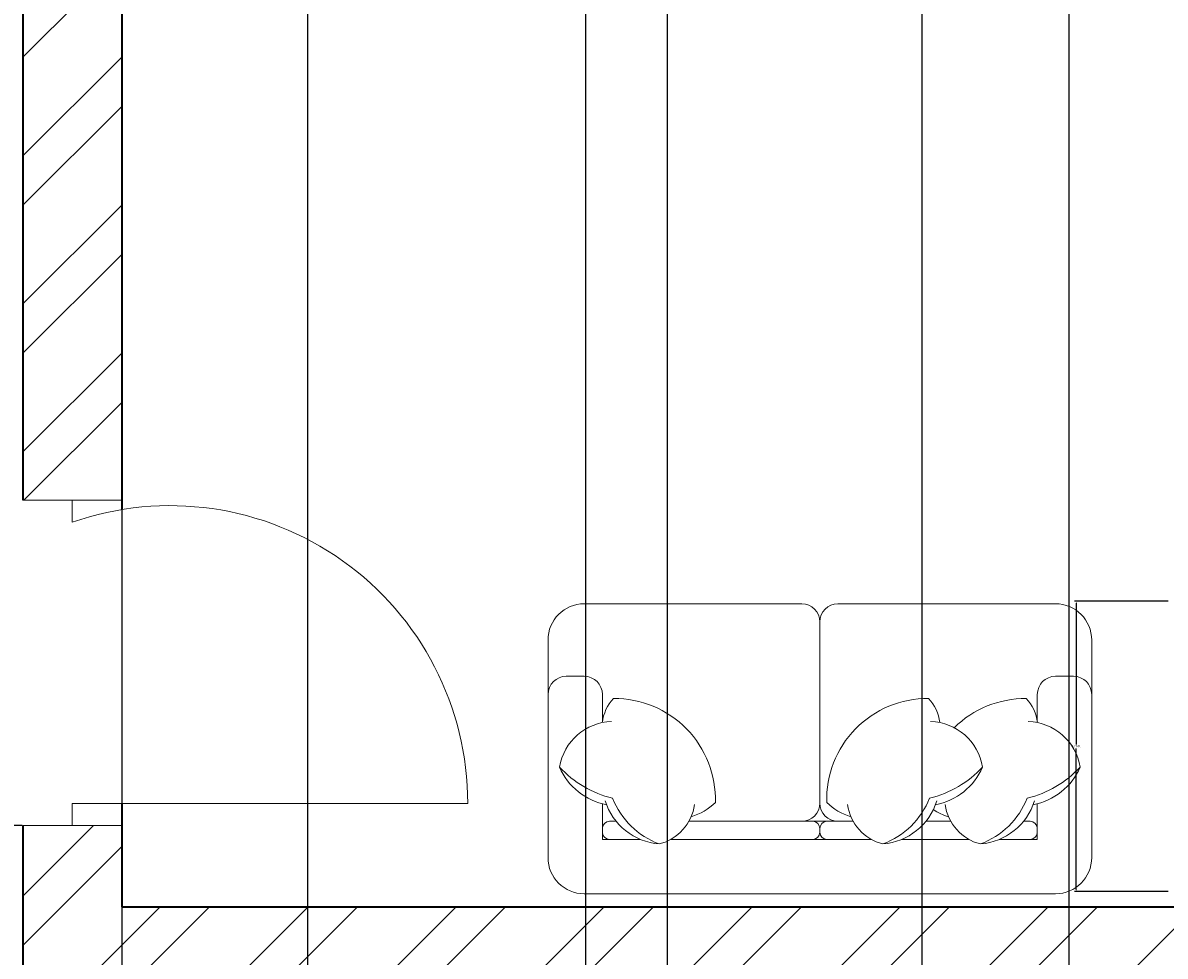
# Model space of a CAD drawing. Units: inches. Extents: x 2552 to 3217, y 1417 to 2737.
# Tile 20 of 25: x 2909 to 3013, y 2392 to 2476. Entities that reach past the tile are written whole.
import ezdxf

# ---------------------------------------------------------------- set-up
doc = ezdxf.new("R2010")
doc.units = ezdxf.units.IN
for name, color, linetype, lineweight in [('A-ANNO-DIMS', 2, 'Continuous', 18), ('A-DOOR', 21, 'Continuous', 18), ('A-FURN', 8, 'Continuous', 13), ('A-WALL', 7, 'Continuous', 35), ('A-WALL-PATT', 217, 'Continuous', 13)]:
    doc.layers.add(name, color=color, linetype=linetype, lineweight=lineweight)
doc.styles.get("Standard").update_dxf_attribs({"font": 'arial.ttf'})
doc.dimstyles.get("Standard").update_dxf_attribs({"dimtxt": 0.18, "dimasz": 0.18, "dimexe": 0.18, "dimexo": 0.0625, "dimgap": 0.09, "dimtad": 0, "dimtih": 1, "dimtoh": 1, "dimdec": 4, "dimzin": 0, "dimdsep": 46, "dimtxsty": 'Standard', "dimcen": 0.09, "dimadec": 0, "dimazin": 0, "dimtfac": 1, "dimtdec": 4, "dimtofl": 0, "dimtmove": 0, "dimatfit": 3, "dimfxl": 1, "dimtolj": 1, "dimtzin": 0, "dimarcsym": 0})

# ---------------------------------------------------------------- blocks, each defined once
blk = doc.blocks.new('*D46')
at = {"layer": 'A-ANNO-DIMS', "color": 0, "lineweight": -2, "transparency": 16777216}
for p, q in [((3013.1, 2423.8), (3004.57, 2423.8)), ((3004.75, 2423.62), (3004.75, 2410.78)), ((3004.75, 2397.59), (3004.75, 2410.42)), ((3013.1, 2397.41), (3004.57, 2397.41))]:
    blk.add_line(p, q, dxfattribs=at)
at = {"layer": 'A-ANNO-DIMS', "color": 0, "transparency": 16777216}
for points in [[(3004.72, 2423.62), (3004.78, 2423.62), (3004.75, 2423.8)], [(3004.72, 2397.59), (3004.78, 2397.59), (3004.75, 2397.41)]]:
    blk.add_solid(points, dxfattribs=at)
at = {"layer": 'Defpoints', "color": 0, "transparency": 16777216}
for p in [(3004.75, 2423.8), (3013.16, 2423.8), (3013.16, 2397.41)]:
    blk.add_point(p, dxfattribs=at)
at = {"layer": 'A-ANNO-DIMS', "color": 0, "transparency": 16777216, "insert": (3004.75, 2410.6), "char_height": 0.18, "attachment_point": 5}
blk.add_mtext('\\A1;26 TYP.', dxfattribs=at)
blk = doc.blocks.new('*D56')
at = {"layer": 'A-ANNO-DIMS', "color": 0, "lineweight": -2, "transparency": 16777216}
for p, q in [((2967.49, 2515.95), (2967.49, 1482.53)), ((2990.69, 2515.95), (2990.69, 1482.53)), ((2967.67, 1482.71), (2978.76, 1482.71)), ((2990.51, 1482.71), (2979.41, 1482.71))]:
    blk.add_line(p, q, dxfattribs=at)
at = {"layer": 'A-ANNO-DIMS', "color": 0, "transparency": 16777216}
for points in [[(2967.67, 1482.74), (2967.67, 1482.68), (2967.49, 1482.71)], [(2990.51, 1482.74), (2990.51, 1482.68), (2990.69, 1482.71)]]:
    blk.add_solid(points, dxfattribs=at)
at = {"layer": 'Defpoints', "color": 0, "transparency": 16777216}
for p in [(2967.49, 2516.01), (2990.69, 2516.01), (2990.69, 1482.71)]:
    blk.add_point(p, dxfattribs=at)
at = {"layer": 'A-ANNO-DIMS', "color": 0, "transparency": 16777216, "insert": (2979.09, 1482.71), "char_height": 0.18, "attachment_point": 5}
blk.add_mtext('\\A1;23.2', dxfattribs=at)
blk = doc.blocks.new('*D57')
at = {"layer": 'A-ANNO-DIMS', "color": 0, "lineweight": -2, "transparency": 16777216}
for p, q in [((3004.08, 2515.95), (3004.08, 1482.53)), ((3036.34, 2515.95), (3036.34, 1482.53)), ((3004.26, 1482.71), (3019.75, 1482.71)), ((3036.16, 1482.71), (3020.68, 1482.71))]:
    blk.add_line(p, q, dxfattribs=at)
at = {"layer": 'A-ANNO-DIMS', "color": 0, "transparency": 16777216}
for points in [[(3004.26, 1482.74), (3004.26, 1482.68), (3004.08, 1482.71)], [(3036.16, 1482.74), (3036.16, 1482.68), (3036.34, 1482.71)]]:
    blk.add_solid(points, dxfattribs=at)
at = {"layer": 'Defpoints', "color": 0, "transparency": 16777216}
for p in [(3004.08, 2516.01), (3036.34, 2516.01), (3036.34, 1482.71)]:
    blk.add_point(p, dxfattribs=at)
at = {"layer": 'A-ANNO-DIMS', "color": 0, "transparency": 16777216, "insert": (3020.21, 1482.71), "char_height": 0.18, "attachment_point": 5}
blk.add_mtext('\\A1;32.255', dxfattribs=at)
blk = doc.blocks.new('*D64')
at = {"layer": 'A-ANNO-DIMS', "color": 0, "lineweight": -2, "transparency": 16777216}
for p, q in [((2646.35, 1551.58), (2646.35, 2709.49)), ((2646.53, 2709.31), (2802.77, 2709.31)), ((2959.93, 2709.31), (2803.69, 2709.31)), ((2960.11, 1551.58), (2960.11, 2709.49))]:
    blk.add_line(p, q, dxfattribs=at)
at = {"layer": 'A-ANNO-DIMS', "color": 0, "transparency": 16777216}
for points in [[(2646.53, 2709.34), (2646.53, 2709.28), (2646.35, 2709.31)], [(2959.93, 2709.34), (2959.93, 2709.28), (2960.11, 2709.31)]]:
    blk.add_solid(points, dxfattribs=at)
at = {"layer": 'Defpoints', "color": 0, "transparency": 16777216}
for p in [(2960.11, 2709.31), (2646.35, 1551.51), (2960.11, 1551.51)]:
    blk.add_point(p, dxfattribs=at)
at = {"layer": 'A-ANNO-DIMS', "color": 0, "transparency": 16777216, "insert": (2803.23, 2709.31), "char_height": 0.18, "attachment_point": 5}
blk.add_mtext('\\A1;313.76', dxfattribs=at)
blk = doc.blocks.new('*D67')
at = {"layer": 'A-ANNO-DIMS', "color": 0, "lineweight": -2, "transparency": 16777216}
for p, q in [((2917.85, 2640.45), (2917.85, 1482.53)), ((2934.77, 2624.73), (2934.77, 1482.53)), ((2918.03, 1482.71), (2925.86, 1482.71)), ((2934.59, 1482.71), (2926.76, 1482.71))]:
    blk.add_line(p, q, dxfattribs=at)
at = {"layer": 'A-ANNO-DIMS', "color": 0, "transparency": 16777216}
for points in [[(2918.03, 1482.74), (2918.03, 1482.68), (2917.85, 1482.71)], [(2934.59, 1482.74), (2934.59, 1482.68), (2934.77, 1482.71)]]:
    blk.add_solid(points, dxfattribs=at)
at = {"layer": 'Defpoints', "color": 0, "transparency": 16777216}
for p in [(2917.85, 2640.51), (2934.77, 2624.79), (2934.77, 1482.71)]:
    blk.add_point(p, dxfattribs=at)
at = {"layer": 'A-ANNO-DIMS', "color": 0, "transparency": 16777216, "insert": (2926.31, 1482.71), "char_height": 0.18, "attachment_point": 5}
blk.add_mtext('\\A1;16.912', dxfattribs=at)
blk = doc.blocks.new('*D69')
at = {"layer": 'A-ANNO-DIMS', "color": 0, "lineweight": -2, "transparency": 16777216}
for p, q in [((2908.79, 2403.41), (2577.37, 2403.41)), ((2577.55, 2403.23), (2577.55, 2395.39)), ((2577.55, 2387.19), (2577.55, 2395.03)), ((2917.79, 2387.01), (2577.37, 2387.01))]:
    blk.add_line(p, q, dxfattribs=at)
at = {"layer": 'A-ANNO-DIMS', "color": 0, "transparency": 16777216}
for points in [[(2577.52, 2403.23), (2577.58, 2403.23), (2577.55, 2403.41)], [(2577.52, 2387.19), (2577.58, 2387.19), (2577.55, 2387.01)]]:
    blk.add_solid(points, dxfattribs=at)
at = {"layer": 'Defpoints', "color": 0, "transparency": 16777216}
for p in [(2577.55, 2403.41), (2908.85, 2403.41), (2917.85, 2387.01)]:
    blk.add_point(p, dxfattribs=at)
at = {"layer": 'A-ANNO-DIMS', "color": 0, "transparency": 16777216, "insert": (2577.55, 2395.21), "char_height": 0.18, "attachment_point": 5}
blk.add_mtext('\\A1;16.4', dxfattribs=at)

msp = doc.modelspace()

# ---------------------------------------------------------------- hatches: boundary and pattern name
at = {"layer": 'A-WALL-PATT'}
h = msp.add_hatch(dxfattribs=at)
h.set_pattern_fill('ANSI32', color=256)
h.paths.add_polyline_path([(2756.676, 2649.5125), (2637.3535, 2649.5125), (2637.3535, 2617.9626), (2641.8535, 2617.9626), (2646.3535, 2617.9626), (2646.3535, 2640.5125), (2724.3535, 2640.5125), (2724.3535, 2520.5125), (2720.299, 2520.5125), (2720.299, 2516.0125), (2733.4075, 2516.0125), (2733.4075, 2518.2213), (2733.4075, 2520.5125), (2728.8535, 2520.5125), (2728.8535, 2640.5125), (2756.676, 2640.5125)])
h.paths.add_polyline_path([(2848.8535, 2649.5125), (2804.676, 2649.5125), (2804.676, 2640.5125), (2839.8535, 2640.5125), (2839.8535, 2598.3517), (2848.8535, 2598.3517)])
h.paths.add_polyline_path([(2646.3535, 2516.0125), (2697.9593, 2516.0125), (2697.9593, 2518.2625), (2697.9593, 2520.5125), (2646.3535, 2520.5125), (2646.3535, 2581.9626), (2637.3535, 2581.9626), (2637.3535, 2364.3298), (2646.3535, 2364.3298), (2646.3535, 2387.0125), (2724.3535, 2387.0125), (2724.3535, 2267.0125), (2721.0443, 2267.0125), (2721.0443, 2262.5125), (2733.7854, 2262.5125), (2733.7854, 2264.7625), (2733.7854, 2267.0125), (2728.8535, 2267.0125), (2728.8535, 2387.0125), (2839.8535, 2387.0125), (2839.8535, 2363.8387), (2848.8535, 2363.8387), (2848.8535, 2403.7415), (2844.3535, 2403.7415), (2839.8535, 2403.7415), (2839.8535, 2396.0125), (2646.3535, 2396.0125)])
h.paths.add_polyline_path([(2848.8535, 2550.3517), (2844.3535, 2550.3517), (2839.8535, 2550.3517), (2839.8535, 2520.5125), (2801.9195, 2520.5125), (2801.9195, 2518.2625), (2801.9195, 2516.0125), (2839.8535, 2516.0125), (2839.8535, 2507.5813), (2848.8535, 2507.5813)], flags=17)
h.paths.add_polyline_path([(2848.8535, 2483.5813), (2844.3535, 2483.5813), (2839.8535, 2483.5813), (2839.8535, 2468.0125), (2773.8535, 2468.0125), (2773.8535, 2516.0125), (2778.1336, 2516.0125), (2778.1336, 2520.5125), (2766.696, 2520.5125), (2766.696, 2518.2625), (2766.696, 2516.0125), (2769.3535, 2516.0125), (2769.3535, 2463.5125), (2839.8535, 2463.5125), (2839.8535, 2431.0782), (2848.8535, 2431.0782)], flags=17)
h.paths.add_polyline_path([(2917.8535, 2569.2764), (2913.3535, 2569.2764), (2908.8535, 2569.2764), (2908.8535, 2433.001), (2917.8535, 2433.001), (2917.8535, 2516.0125), (2967.486, 2516.0125), (2967.486, 2520.5125), (2917.8535, 2520.5125)])
h.paths.add_polyline_path([(3000.3535, 2640.5125), (2995.8535, 2640.5125), (2995.8535, 2520.5125), (2990.688, 2520.5125), (2990.688, 2516.0125), (3004.0844, 2516.0125), (3004.0844, 2518.2625), (3004.0844, 2520.5125), (3000.3535, 2520.5125)])
h.paths.add_polyline_path([(3120.3535, 2561.3689), (3115.8535, 2561.3689), (3111.3535, 2561.3689), (3111.3535, 2520.5125), (3070.9814, 2520.5125), (3070.9814, 2518.2625), (3070.9814, 2516.0125), (3111.3535, 2516.0125), (3111.3535, 2505.1841), (3120.3535, 2505.1841)])
h.paths.add_polyline_path([(3120.3535, 2481.1841), (3115.8535, 2481.1841), (3111.3535, 2481.1841), (3111.3535, 2468.0125), (3045.3535, 2468.0125), (3045.3535, 2516.0125), (3048.9787, 2516.0125), (3048.9787, 2520.5125), (3036.3395, 2520.5125), (3036.3395, 2516.0125), (3040.8535, 2516.0125), (3040.8535, 2463.5125), (3111.3535, 2463.5125), (3111.3535, 2396.0125), (2917.8535, 2396.0125), (2917.8535, 2403.4124), (2913.3535, 2403.4124), (2908.8535, 2403.4124), (2908.8535, 2182.5756), (2917.8535, 2182.5756), (2917.8535, 2262.5125), (2968.001, 2262.5125), (2968.001, 2264.7625), (2968.001, 2267.0125), (2917.8535, 2267.0125), (2917.8535, 2387.0125), (3111.3535, 2387.0125), (3111.3535, 2352.2435), (3120.3535, 2352.2435)])
h.paths.add_polyline_path([(3120.3535, 2304.2435), (3115.8535, 2304.2435), (3111.3535, 2304.2435), (3111.3535, 2267.0125), (3073.8616, 2267.0125), (3073.8616, 2264.7625), (3073.8616, 2262.5125), (3111.3535, 2262.5125), (3111.3535, 2252.376), (3120.3535, 2252.376)], flags=17)
h.paths.add_polyline_path([(3120.3535, 2228.376), (3115.8535, 2228.376), (3111.3535, 2228.376), (3111.3535, 2214.5125), (3045.3535, 2214.5125), (3045.3535, 2262.5125), (3049.3096, 2262.5125), (3049.3096, 2267.0125), (3035.0125, 2267.0125), (3035.0125, 2262.5125), (3040.8535, 2262.5125), (3040.8535, 2210.0125), (3111.3535, 2210.0125), (3111.3535, 2142.5125), (2917.8535, 2142.5125), (2917.8535, 2150.2408), (2913.3535, 2150.2408), (2908.8535, 2150.2408), (2908.8535, 1924.9905), (2917.8535, 1924.9905), (2917.8535, 2009.0125), (2971.959, 2009.0125), (2971.959, 2011.2625), (2971.959, 2013.5125), (2917.8535, 2013.5125), (2917.8535, 2133.5125), (2995.8535, 2133.5125), (2995.8535, 2013.5125), (2992.1797, 2013.5125), (2992.1797, 2009.0125), (3004.3344, 2009.0125), (3004.3344, 2011.2625), (3004.3344, 2013.5125), (3000.3535, 2013.5125), (3000.3535, 2133.5125), (3111.3535, 2133.5125), (3111.3535, 2115.0291), (3120.3535, 2115.0291)])
h.paths.add_polyline_path([(3000.3535, 2387.0125), (2995.8535, 2387.0125), (2995.8535, 2267.0125), (2991.3326, 2267.0125), (2991.3326, 2262.5125), (3004.1044, 2262.5125), (3004.1044, 2264.7625), (3004.1044, 2267.0125), (3000.3535, 2267.0125)], flags=17)
h.paths.add_polyline_path([(3120.3535, 1973.2388), (3115.8535, 1973.2388), (3111.3535, 1973.2388), (3111.3535, 1961.0125), (3045.3535, 1961.0125), (3045.3535, 2009.0125), (3048.9101, 2009.0125), (3048.9101, 2013.5125), (3037.105, 2013.5125), (3037.105, 2011.2625), (3037.105, 2009.0125), (3040.8535, 2009.0125), (3040.8535, 1956.5125), (3111.3535, 1956.5125), (3111.3535, 1889.0125), (2917.8535, 1889.0125), (2917.8535, 1895.7215), (2913.3535, 1895.7215), (2908.8535, 1895.7215), (2908.8535, 1844.2217), (2917.8535, 1844.2217), (2917.8535, 1880.0125), (3111.3535, 1880.0125), (3111.3535, 1846.9541), (3120.3535, 1846.9541)])
h.paths.add_polyline_path([(3120.3535, 2067.0291), (3111.3535, 2067.0291), (3111.3535, 2013.5125), (3071.3001, 2013.5125), (3071.3001, 2009.0125), (3111.3535, 2009.0125), (3111.3535, 1997.2388), (3120.3535, 1997.2388)], flags=0)
h.paths.add_polyline_path([(3120.3535, 1798.9541), (3115.8535, 1798.9541), (3111.3535, 1798.9541), (3111.3535, 1760.0125), (3071.2497, 1760.0125), (3071.2497, 1757.7625), (3071.2497, 1755.5125), (3111.3535, 1755.5125), (3111.3535, 1746.162), (3120.3535, 1746.2478)])
h.paths.add_polyline_path([(3120.3535, 1722.2049), (3111.3535, 1722.2049), (3111.3535, 1707.5125), (3045.3535, 1707.5125), (3045.3535, 1755.5125), (3048.6624, 1755.5125), (3048.6624, 1760.0125), (3035.3703, 1760.0125), (3035.3703, 1755.5125), (3040.8535, 1755.5125), (3040.8535, 1703.0125), (3111.3535, 1703.0125), (3111.3535, 1635.5125), (2917.8535, 1635.5125), (2917.8535, 1643.1366), (2913.3535, 1643.1366), (2908.8535, 1643.1366), (2908.8535, 1626.5125), (3120.3535, 1626.5125)])
h.paths.add_polyline_path([(2917.8535, 1755.5125), (2973.2287, 1755.5125), (2973.2287, 1757.7625), (2973.2287, 1760.0125), (2917.8535, 1760.0125), (2917.8535, 1808.2217), (2913.3535, 1808.2217), (2908.8535, 1808.2217), (2908.8535, 1676.1665), (2917.8535, 1676.1665)])
h.paths.add_polyline_path([(3000.3535, 1880.0125), (2995.8535, 1880.0125), (2995.8535, 1760.0125), (2992.9329, 1760.0125), (2992.9329, 1755.5125), (3003.8766, 1755.5125), (3003.8766, 1757.7625), (3003.8766, 1760.0125), (3000.3535, 1760.0125)])
h.paths.add_polyline_path([(2848.8535, 1896.6971), (2844.3535, 1896.6971), (2839.8535, 1896.6971), (2839.8535, 1889.0125), (2646.3535, 1889.0125), (2646.3535, 2009.0125), (2700.5253, 2009.0125), (2700.5253, 2011.2625), (2700.5253, 2013.5125), (2646.3535, 2013.5125), (2646.3535, 2053.1812), (2641.8535, 2053.1812), (2637.3535, 2053.1812), (2637.3535, 1836.254), (2646.3535, 1836.254), (2646.3535, 1880.0125), (2724.3535, 1880.0125), (2724.3535, 1760.0125), (2721.2473, 1760.0125), (2721.2473, 1755.5125), (2731.9187, 1755.5125), (2731.9187, 1757.7625), (2731.9187, 1760.0125), (2728.8535, 1760.0125), (2728.8535, 1880.0125), (2839.8535, 1880.0125), (2839.8535, 1840.3813), (2848.8535, 1840.3813)])
h.paths.add_polyline_path([(2848.8535, 1792.3813), (2844.3535, 1792.3813), (2839.8535, 1792.3813), (2839.8535, 1760.0125), (2797.8845, 1760.0125), (2797.8845, 1755.5125), (2839.8535, 1755.5125), (2839.8535, 1743.3688), (2844.3535, 1743.3688), (2848.8535, 1743.3688)], flags=0)
h.paths.add_polyline_path([(2848.8535, 1719.3688), (2844.3535, 1719.3688), (2839.8535, 1719.3688), (2839.8535, 1707.5125), (2773.8535, 1707.5125), (2773.8535, 1755.5125), (2777.716, 1755.5125), (2777.716, 1760.0125), (2760.9247, 1760.0125), (2760.9247, 1757.9721), (2760.9247, 1755.5125), (2769.3535, 1755.5125), (2769.3535, 1703.0125), (2839.8535, 1703.0125), (2839.8535, 1673.0277), (2848.8535, 1672.9407)], flags=0)
h.paths.add_polyline_path([(2646.3535, 1755.5125), (2702.9171, 1755.5125), (2702.9171, 1757.7625), (2702.9171, 1760.0125), (2646.3535, 1760.0125), (2646.3535, 1800.254), (2641.8535, 1800.254), (2637.3535, 1800.254), (2637.3535, 1626.5125), (2848.8535, 1626.5125), (2848.8535, 1643.1187), (2844.3535, 1643.1187), (2839.8535, 1643.1187), (2839.8535, 1635.5125), (2646.3535, 1635.5125)])
h.paths.add_polyline_path([(2848.8535, 2148.8427), (2844.3535, 2148.8427), (2839.8535, 2148.8427), (2839.8535, 2142.5125), (2646.3535, 2142.5125), (2646.3535, 2262.5125), (2701.3562, 2262.5125), (2701.3562, 2264.7625), (2701.3562, 2267.0125), (2646.3535, 2267.0125), (2646.3535, 2328.3298), (2637.3535, 2328.3298), (2637.3535, 2089.1812), (2646.3535, 2089.1812), (2646.3535, 2133.5125), (2839.8535, 2133.5125), (2839.8535, 2097.5966), (2848.8535, 2097.5966)])
h.paths.add_polyline_path([(2728.8535, 2133.5125), (2724.3535, 2133.5125), (2724.3535, 2013.5125), (2719.6039, 2013.5125), (2719.6039, 2009.0125), (2732.5784, 2009.0125), (2732.5784, 2011.2625), (2732.5784, 2013.5125), (2728.8535, 2013.5125)])
h.paths.add_polyline_path([(2848.8535, 1970.0557), (2844.3535, 1970.0557), (2839.8535, 1970.0557), (2839.8535, 1961.0125), (2773.8535, 1961.0125), (2773.8535, 2009.0125), (2777.3388, 2009.0125), (2777.3388, 2013.5125), (2764.7681, 2013.5125), (2764.7681, 2009.0125), (2769.3535, 2009.0125), (2769.3535, 1956.5125), (2839.8535, 1956.5125), (2839.8535, 1924.7199), (2848.8535, 1924.7199)], flags=17)
h.paths.add_polyline_path([(2848.8535, 2049.5966), (2844.3535, 2049.5966), (2839.8535, 2049.5966), (2839.8535, 2013.5125), (2798.198, 2013.5125), (2798.198, 2011.2625), (2798.198, 2009.0125), (2839.8535, 2009.0125), (2839.8535, 1994.0557), (2848.8535, 1994.0557)], flags=17)
h.paths.add_polyline_path([(2848.8535, 2315.8387), (2839.8535, 2315.8387), (2839.8535, 2267.0125), (2799.3375, 2267.0125), (2799.3375, 2264.7625), (2799.3375, 2262.5125), (2839.8535, 2262.5125), (2839.8535, 2253.2843), (2848.8535, 2253.2843)], flags=17)
h.paths.add_polyline_path([(2848.8535, 2229.2843), (2839.8535, 2229.2843), (2839.8535, 2177.6936), (2848.8535, 2177.6936)], flags=17)
h.paths.add_polyline_path([(2839.8535, 2214.5125), (2773.8535, 2214.5125), (2773.8535, 2262.5125), (2777.6984, 2262.5125), (2777.6984, 2267.0125), (2763.8226, 2267.0125), (2763.8226, 2262.5125), (2769.3535, 2262.5125), (2769.3535, 2210.0125), (2839.8535, 2210.0125)], flags=17)
h.paths.add_polyline_path([(3050.32, 2520.2817), (3088.9114, 2520.2817), (3088.9114, 2538.939), (3050.32, 2538.939)], flags=9)

# ---------------------------------------------------------------- linework, layer by layer
at = {"layer": 'A-DOOR'}
for p, q in [((2908.8535, 2433.001), (2917.8535, 2433.001)), ((2917.8535, 2433.001), (2913.3535, 2433.001)), ((2913.3535, 2433.001), (2913.3535, 2431.001)), ((2913.3535, 2403.4124), (2913.3535, 2405.4124)), ((2913.3535, 2405.4124), (2949.3535, 2405.4124)), ((2908.8535, 2403.4124), (2917.8535, 2403.4124)), ((2917.8535, 2403.4124), (2913.3535, 2403.4124)), ((2913.3535, 2403.4124), (2913.3535, 2403.4124)), ((2917.8535, 2403.4124), (2917.8535, 2403.4124))]:
    msp.add_line(p, q, dxfattribs=at)
msp.add_arc((2922.2594, 2405.4124), 27.0941, 0, 109.189918, dxfattribs=at)
at = {"layer": 'A-FURN', "ltscale": 0.03}
msp.add_lwpolyline([(2979.7543, 2423.5767, -0.41421356), (2981.4039, 2421.9272, -0.41421356), (2983.0534, 2423.5767), (3002.8482, 2423.5767, -0.41421356), (3006.1473, 2420.2776), (3006.1473, 2400.4828, -0.41421356), (3002.8482, 2397.1837), (2959.9596, 2397.1837, -0.41421356), (2956.6604, 2400.4828), (2956.6604, 2420.2776, -0.41421356), (2959.9596, 2423.5767), (2979.7543, 2423.5767, -0.41421356), (2981.4039, 2421.9272, -0.41421356), (2983.0534, 2423.5767)], format="xyb", dxfattribs=at)
at = {"layer": 'A-FURN'}
for points in [[(2979.7543, 2403.782, 0.41421356), (2981.4039, 2405.4315), (2981.4039, 2421.9272, 0.41421356)], [(2983.0534, 2403.782, -0.41421356), (2981.4039, 2405.4315), (2981.4039, 2421.9272, -0.41421356)], [(2956.6604, 2415.3289, -0.41421356), (2958.31, 2416.9785), (2959.9596, 2416.9785, -0.41421356), (2961.6091, 2415.3289), (2961.6091, 2412.7731)], [(3001.1986, 2412.7731), (3001.1986, 2415.3289, -0.41421356), (3002.8482, 2416.9785), (3004.4978, 2416.9785, -0.41421356), (3006.1473, 2415.3289)], [(2961.6055, 2412.7724, -0.16554063), (2962.626, 2414.9519, -0.42598917), (2971.8903, 2405.5021, -0.12152332), (2969.6911, 2404.1996, 7.11546429)], [(2992.3161, 2412.7724, 0.16554063), (2991.2956, 2414.9519, 0.42598917), (2982.0314, 2405.5021, 0.12152332), (2984.2305, 2404.1996, -7.11546429)], [(3001.2022, 2412.7724, 0.16554063), (3000.1818, 2414.9519, 0.20023115), (2993.6336, 2412.2975, 0.12152332)], [(2962.4369, 2412.873, 0.35677236), (2957.7103, 2408.715, 0.24954205), (2961.9931, 2405.2886, -9.61688035)], [(2991.4847, 2412.873, -0.35677236), (2996.2114, 2408.715, -0.24954205), (2991.9286, 2405.2886, 9.61688035)], [(3000.3708, 2412.873, -0.35677236), (3005.0975, 2408.715, -0.24954205), (3000.8147, 2405.2886, 9.61688035)], [(2957.7103, 2408.715, 0.14772988), (2962.5315, 2405.8801, 0.21334276), (2966.7855, 2401.7222, 0.17866181)], [(2996.2114, 2408.715, -0.14772988), (2991.3902, 2405.8801, -0.21334276), (2987.1362, 2401.7222, -0.17866181)], [(3005.0975, 2408.715, -0.14772988), (3000.2763, 2405.8801, -0.21334276), (2996.0223, 2401.7222, -0.17866181)], [(2961.8654, 2405.6542, 0.30666349), (2966.7855, 2401.7222, 0.30632997), (2969.9996, 2405.3131, -0.87284716)], [(2979.7543, 2403.782, 0.41421356), (2981.4039, 2405.4315)], [(2983.0534, 2403.782, -0.41421356), (2981.4039, 2405.4315)], [(2992.0562, 2405.6542, -0.30666349), (2987.1362, 2401.7222, -0.30632997), (2983.922, 2405.3131, 0.87284716)], [(3000.9423, 2405.6542, -0.30666349), (2996.0223, 2401.7222, -0.30632997), (2992.8082, 2405.3131, 0.87284716)], [(2997.7284, 2402.1324), (3001.1986, 2402.1324), (3001.1986, 2405.3742, -0.41421356)], [(2991.7337, 2404.8445, 0.07186538), (2993.1166, 2404.1996, -7.11546429)], [(2962.8679, 2403.782), (2962.2689, 2403.782, 0.41421356), (2961.6091, 2403.1221), (2961.6091, 2402.7922, 0.41421356), (2962.2689, 2402.1324)], [(2967.8236, 2402.1324), (2980.7441, 2402.1324, 0.41421356), (2981.4039, 2402.7922), (2981.4039, 2403.1221, 0.41421356), (2980.7441, 2403.782), (2969.4846, 2403.782, 0.41421356)], [(2986.098, 2402.1324), (2982.0637, 2402.1324, -0.41421356), (2981.4039, 2402.7922), (2981.4039, 2403.1221, -0.41421356), (2982.0637, 2403.782), (2984.437, 2403.782, -0.41421356)], [(2991.0537, 2403.782), (2993.3231, 2403.782, -0.41421356)], [(2999.9398, 2403.782), (3000.5388, 2403.782, -0.41421356), (3001.1986, 2403.1221), (3001.1986, 2402.7922, -0.41421356), (3000.5388, 2402.1324)], [(2962.2689, 2402.1324), (2965.0793, 2402.1324, 0.41421356)], [(2994.9841, 2402.1324), (2988.8423, 2402.1324, -0.41421356)], [(3000.5388, 2402.1324), (2997.7284, 2402.1324, -0.41421356)]]:
    msp.add_lwpolyline(points, format="xyb", dxfattribs=at)
for points in [[(2961.6091, 2405.3742), (2961.6091, 2402.1324), (2965.0793, 2402.1324)], [(2967.8236, 2402.1324), (2986.098, 2402.1324)], [(2988.8423, 2402.1324), (2994.9841, 2402.1324)]]:
    msp.add_lwpolyline(points, dxfattribs=at)
msp.add_lwpolyline([(2980.7441, 2402.1324), (2982.0637, 2402.1324, -0.41421356), (2981.4039, 2402.7922), (2981.4039, 2403.1221, -0.41421356), (2982.0637, 2403.782), (2980.7441, 2403.782, -0.41421356), (2981.4039, 2403.1221), (2981.4039, 2402.7922, -0.41421356)], format="xyb", close=True, dxfattribs=at)
at = {"layer": 'A-WALL'}
for p, q in [((2908.8535, 2569.2764), (2908.8535, 2433.001)), ((2917.8535, 2516.0125), (2917.8535, 2432.1459)), ((2917.8535, 2405.4124), (2917.8535, 2396.0125)), ((2908.8535, 2403.4124), (2908.8535, 2182.5756)), ((2917.8535, 2396.0125), (3111.3535, 2396.0125))]:
    msp.add_line(p, q, dxfattribs=at)

# ---------------------------------------------------------------- dimensions: what is measured, and where the dimension line sits
at = {"layer": 'A-ANNO-DIMS'}
for base, p1, p2, override, picture, middle in [((2960.1089, 2709.3125), (2646.3535, 1551.5125), (2960.1089, 1551.5125), {"dimdec": 2, "dimlfac": 1, "dimrnd": 0, "dimzin": 0, "dimdsep": 46, "dimlunit": 2}, '*D64', (2803.2312, 2709.3125)), ((2934.7654, 1482.7125), (2917.8535, 2640.5125), (2934.7654, 2624.7942), {"dimdec": 3, "dimlfac": 1, "dimrnd": 0, "dimzin": 0, "dimdsep": 46, "dimlunit": 2}, '*D67', (2926.3094, 1482.7125)), ((2990.688, 1482.7125), (2967.486, 2516.0125), (2990.688, 2516.0125), {"dimdec": 1, "dimlfac": 1, "dimrnd": 0, "dimzin": 0, "dimdsep": 46, "dimlunit": 2}, '*D56', (2979.087, 1482.7125)), ((3036.3395, 1482.7125), (3004.0844, 2516.0125), (3036.3395, 2516.0125), {"dimdec": 3, "dimlfac": 1, "dimrnd": 0, "dimzin": 0, "dimdsep": 46, "dimlunit": 2}, '*D57', (3020.212, 1482.7125))]:
    dim = msp.add_linear_dim(base=base, p1=p1, p2=p2, dimstyle='Standard', override=override, dxfattribs=at)
    dim.commit()
    dim.dimension.update_dxf_attribs({"geometry": picture, "text_midpoint": middle})
dim = msp.add_linear_dim(base=(3004.746, 2423.7983), p1=(3013.1588, 2397.4053), p2=(3013.1588, 2423.7983), angle=90, text='<> TYP.', dimstyle='Standard', override={"dimdec": 0, "dimlfac": 1, "dimrnd": 0, "dimzin": 0, "dimdsep": 46, "dimlunit": 2}, dxfattribs=at)
dim.commit()
dim.dimension.update_dxf_attribs({"geometry": '*D46', "text_midpoint": (3004.746, 2410.6018)})
dim = msp.add_linear_dim(base=(2577.5535, 2403.4124), p1=(2917.8535, 2387.0125), p2=(2908.8535, 2403.4124), angle=90, dimstyle='Standard', override={"dimdec": 1, "dimlfac": 1, "dimrnd": 0, "dimzin": 0, "dimdsep": 46, "dimlunit": 2}, dxfattribs=at)
dim.commit()
dim.dimension.update_dxf_attribs({"geometry": '*D69', "text_midpoint": (2577.5535, 2395.2125)})

doc.saveas('drawing.dxf')
